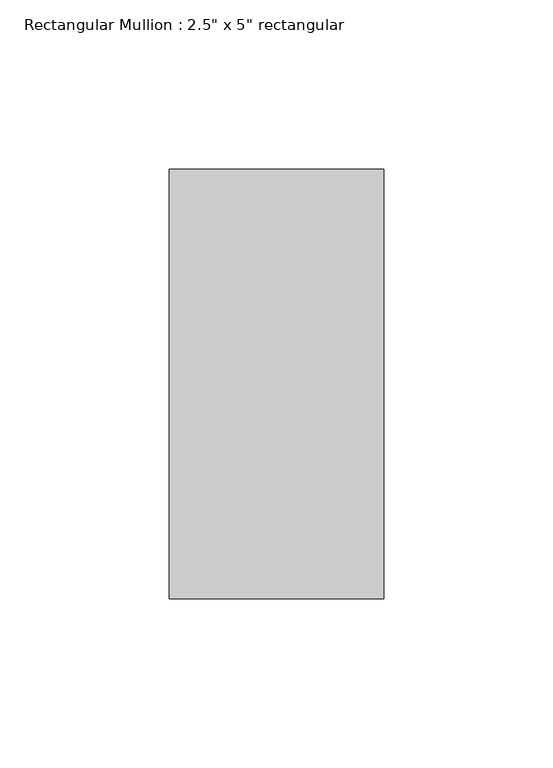
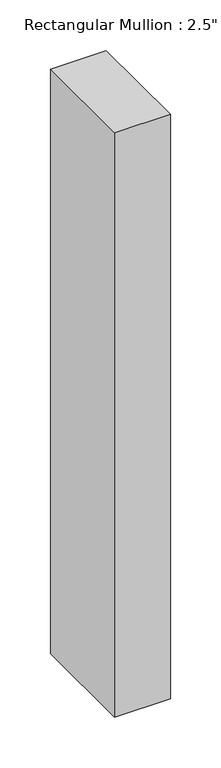
"""IFC4 building model written with IfcOpenShell, lengths in millimetres: member geometry."""

from ifc_helpers import new_model, si_unit, frame, origin, place, context, project, spatial, polyline, outline, extrude, source, transform, mapped, element, save


def member_b956c4f6(model_context):
    return source(origin(), model_context, "Body", "SweptSolid", [
        extrude(outline(polyline([(0.0, 63.5), (0.0, -63.5), (-63.5, -63.5), (-63.5, 63.5), (0.0, 63.5)])), frame((0.0, 0.0, -704.85), z_axis=(0.0, 0.0, 1.0), x_axis=(1.0, 0.0, 0.0)), (0.0, 0.0, 1.0), 704.85),
    ])


if __name__ == "__main__":
    model = new_model("IFC4")
    model_context = context("Model", 3, world=origin())
    ifc_project = project(units=[si_unit("LENGTHUNIT", "METRE", prefix="MILLI")], contexts=[model_context])
    site = spatial("IfcSite", under=ifc_project)
    building = spatial("IfcBuilding", under=site)
    placement = place(None, origin())
    member_shape = member_b956c4f6(model_context)
    element("IfcMember", 1, ObjectType="Rectangular Mullion : 2.5\" x 5\" rectangular", at=placement, inside=building, context=model_context, shape_type="MappedRepresentation", body=[
        mapped(member_shape, transform((0.0, 0.0, 0.0), x_axis=(1.0, 0.0, 0.0), y_axis=(0.0, 1.0, 0.0), z_axis=(0.0, 0.0, 1.0))),
    ])
    save(model, "model.ifc")

# Revit data of these elements
# Type "Rectangular Mullion : 2.5\" x 5\" rectangular"
#   built-in parameter 1007304 = 0.416667 (stored number, unit not read)
#   built-in parameter 1007301 = 0.104167 (stored number, unit not read)
#   built-in parameter 1007300 = 0.104167 (stored number, unit not read)
# Element 1 (IfcMember, "Rectangular Mullion : 2.5\" x 5\" rectangular")
#   Materials on its faces: "Aluminum"
# Materials
#   "Aluminum": class "Metal", colour RGB 247 247 247, transparency 0, Description = "Aluminum 6061", Cost = 0
